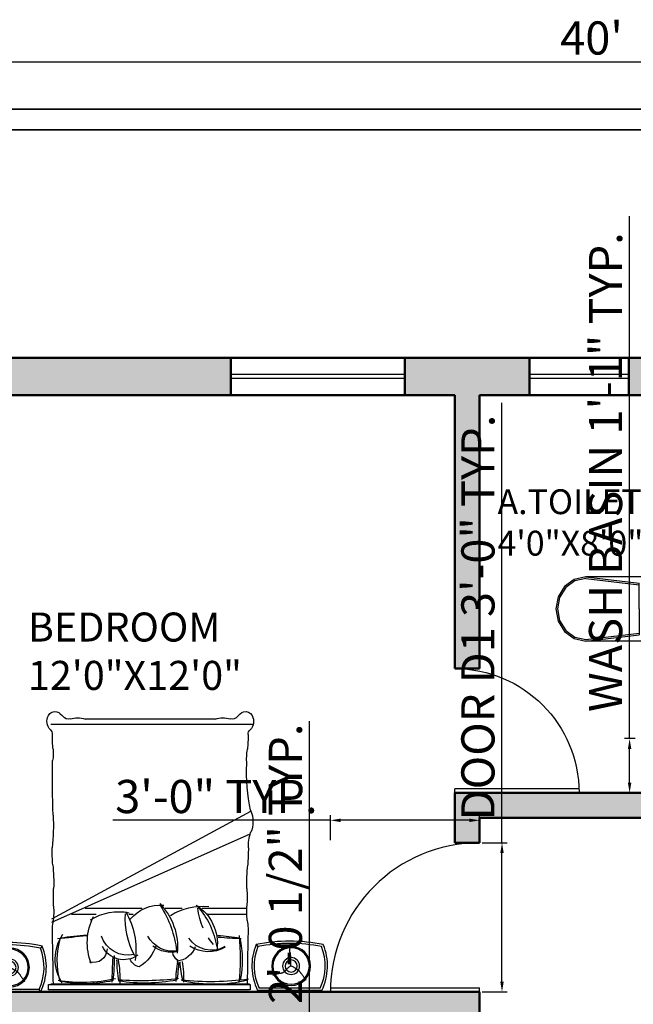
# Model space of a CAD drawing. Units: inches. Extents: x 3008 to 4088, y 1255 to 2137.
# Tile 27 of 30: x 3705 to 3853, y 1794 to 2031. Entities that reach past the tile are written whole.
import ezdxf

# ---------------------------------------------------------------- set-up
doc = ezdxf.new("R2010")
doc.units = ezdxf.units.IN
for name, color, linetype, lineweight in [('A-ANNO-DIMS', 2, 'Continuous', 18), ('A-AREA-IDEN', 7, 'Continuous', 18), ('A-DOOR', 4, 'Continuous', 25), ('A-FLOR-FIXT', 8, 'Continuous', 18), ('A-FURN', 8, 'Continuous', 18), ('A-GLAZ', 4, 'Continuous', 25), ('A-WALL', 7, 'Continuous', 50), ('A-WALL-PATT', 8, 'Continuous', 13), ('C-PROP', 1, 'Continuous', 35)]:
    doc.layers.add(name, color=color, linetype=linetype, lineweight=lineweight)
doc.layers.add('SANTEH', color=7, linetype='Continuous')
doc.layers.add('TEFRİŞ', color=11, linetype='Continuous')
doc.styles.get("Standard").update_dxf_attribs({"font": 'arial.ttf'})
doc.dimstyles.new('ISO-25', dxfattribs={"dimtxt": 8, "dimasz": 2.5, "dimexe": 1.25, "dimexo": 0.625, "dimtad": 1, "dimdec": 1, "dimlunit": 3, "dimtxsty": 'Standard', "dimcen": 2.5, "dimadec": 0, "dimazin": 0, "dimtfac": 1, "dimtdec": 1, "dimtmove": 0, "dimatfit": 3, "dimfxl": 1, "dimarcsym": 0})

# ---------------------------------------------------------------- blocks, each defined once
blk = doc.blocks.new('*D31')
at = {"layer": 'A-ANNO-DIMS', "color": 0, "lineweight": -2, "transparency": 16777216}
for p, q in [((3602.94, 2010.35), (3602.94, 2022.41)), ((4082.94, 2010.35), (4082.94, 2022.41)), ((3605.44, 2021.16), (4080.44, 2021.16))]:
    blk.add_line(p, q, dxfattribs=at)
at = {"layer": 'A-ANNO-DIMS', "color": 0, "transparency": 16777216}
for points in [[(3605.44, 2021.58), (3605.44, 2020.74), (3602.94, 2021.16)], [(4080.44, 2021.58), (4080.44, 2020.74), (4082.94, 2021.16)]]:
    blk.add_solid(points, dxfattribs=at)
at = {"layer": 'Defpoints', "color": 0, "transparency": 16777216}
for p in [(4082.94, 2021.16), (3602.94, 2009.72), (4082.94, 2009.72)]:
    blk.add_point(p, dxfattribs=at)
at = {"layer": 'A-ANNO-DIMS', "color": 0, "transparency": 16777216, "insert": (3842.94, 2025.87), "char_height": 8, "attachment_point": 5}
blk.add_mtext("40'", dxfattribs=at)
blk = doc.blocks.new('D2')
for p, q in [((1722.5, 1505.46), (1722.5, 1475.46)), ((1723.5, 1505.46), (1723.5, 1475.46)), ((1722.5, 1475.46), (1723.5, 1475.46))]:
    blk.add_line(p, q)
blk.add_arc((1722.5, 1475.46), 30, 0, 90)
blk = doc.blocks.new('D1')
for p, q in [((1805.96, 1500.36), (1805.96, 1464.36)), ((1806.96, 1500.36), (1806.96, 1464.36)), ((1805.96, 1464.36), (1806.96, 1464.36))]:
    blk.add_line(p, q)
blk.add_arc((1805.96, 1464.36), 36, 0, 90)
blk = doc.blocks.new('WC 2 Symb_109')
at = {"layer": 'SANTEH'}
for p, q in [((0, 0), (0, 380)), ((0, 380), (132.4, 380)), ((153.6, 364.9), (506.8, 364.9)), ((506.3, 364.9), (215.7, 330.9)), ((506.3, 356), (215.7, 322)), ((215.7, 190), (215.7, 330.9)), ((215.7, 190), (215.7, 49.1)), ((506.3, 24), (215.7, 58)), ((153.8, 15.1), (506.8, 15.1)), ((506.3, 15.1), (215.7, 49.1)), ((0, 0), (132.4, 0))]:
    blk.add_line(p, q, dxfattribs=at)
for points in [[(154.6, 360.1), (153.9, 364.1), (152.3, 367.9), (150.2, 371.3), (147.4, 374.3), (144.1, 376.7), (140.5, 378.5), (136.5, 379.6), (132.4, 380)], [(154.6, 19.7), (158.6, 62.1), (161.4, 104.7), (163.1, 147.3), (163.7, 189.9), (163.1, 232.5), (161.4, 275.1), (158.6, 317.7), (154.6, 360.1)], [(506.3, 24), (565.5, 36.6), (615.7, 72.6), (649.2, 126.5), (661, 190), (649.2, 253.5), (615.7, 307.4), (565.5, 343.4), (506.3, 356)], [(506.8, 15.1), (569.2, 28.4), (622.2, 66.3), (657.6, 123.1), (670, 190), (657.6, 256.9), (622.2, 313.7), (569.2, 351.6), (506.8, 364.9)], [(132.4, 0), (136.5, 0.4), (140.4, 1.5), (144.1, 3.2), (147.3, 5.6), (150.1, 8.6), (152.3, 12), (153.8, 15.7), (154.6, 19.7)]]:
    blk.add_lwpolyline(points, dxfattribs=at)
blk.add_lwpolyline([(83.6, 208.5), (70.4, 203.1), (64.9, 190), (70.4, 176.9), (83.6, 171.5), (96.8, 176.9), (102.2, 190), (96.8, 203.1)], close=True, dxfattribs=at)
blk = doc.blocks.new('BED')
at = {"layer": 'TEFRİŞ'}
for p, q in [((2114.88, 1835.66), (2129.12, 1835.66)), ((2115.2, 1835.15), (2128.8, 1835.15)), ((2130.81, 1834.34), (2130.81, 1835.55)), ((2175.56, 1834.34), (2130.81, 1834.34)), ((2130.91, 1835.55), (2175.56, 1835.55)), ((2175, 1834.19), (2130.91, 1834.19)), ((2175.56, 1835.55), (2175.56, 1834.34)), ((2177.29, 1835.98), (2177.61, 1835.47)), ((2177.29, 1835.98), (2191.52, 1835.98)), ((2177.61, 1835.47), (2191.2, 1835.47)), ((2191.2, 1835.47), (2191.52, 1835.98)), ((2118.49, 1833.2), (2118.34, 1833.38)), ((2118.49, 1833.2), (2118.34, 1833.38)), ((2118.63, 1833.03), (2118.49, 1833.2)), ((2118.63, 1833.03), (2118.49, 1833.2)), ((2118.75, 1832.88), (2118.63, 1833.03)), ((2118.75, 1832.88), (2118.63, 1833.03)), ((2118.86, 1832.74), (2118.75, 1832.88)), ((2118.86, 1832.74), (2118.75, 1832.88)), ((2118.95, 1832.61), (2118.86, 1832.74)), ((2118.95, 1832.61), (2118.86, 1832.74)), ((2119.04, 1832.48), (2118.95, 1832.61)), ((2119.04, 1832.48), (2118.95, 1832.61)), ((2119.12, 1832.37), (2119.04, 1832.48)), ((2119.12, 1832.37), (2119.04, 1832.48)), ((2119.19, 1832.26), (2119.12, 1832.37)), ((2119.19, 1832.26), (2119.12, 1832.37)), ((2119.26, 1832.16), (2119.19, 1832.26)), ((2119.26, 1832.16), (2119.19, 1832.26)), ((2119.32, 1832.06), (2119.26, 1832.16)), ((2119.32, 1832.06), (2119.26, 1832.16)), ((2119.39, 1831.97), (2119.32, 1832.06)), ((2119.39, 1831.97), (2119.32, 1832.06)), ((2119.45, 1831.89), (2119.39, 1831.97)), ((2119.45, 1831.89), (2119.39, 1831.97)), ((2124.49, 1831.94), (2124.56, 1831.95)), ((2124.49, 1831.94), (2124.56, 1831.95)), ((2124.56, 1831.95), (2124.64, 1831.96)), ((2124.56, 1831.95), (2124.64, 1831.96)), ((2124.64, 1831.96), (2124.71, 1831.98)), ((2124.64, 1831.96), (2124.71, 1831.98)), ((2124.71, 1831.98), (2124.79, 1831.99)), ((2124.71, 1831.98), (2124.79, 1831.99)), ((2124.79, 1831.99), (2124.87, 1832.01)), ((2124.79, 1831.99), (2124.87, 1832.01)), ((2124.87, 1832.01), (2124.96, 1832.03)), ((2124.87, 1832.01), (2124.96, 1832.03)), ((2124.96, 1832.03), (2125.05, 1832.05)), ((2124.96, 1832.03), (2125.05, 1832.05)), ((2125.05, 1832.05), (2125.14, 1832.08)), ((2125.05, 1832.05), (2125.14, 1832.08)), ((2125.14, 1832.08), (2125.23, 1832.11)), ((2125.14, 1832.08), (2125.23, 1832.11)), ((2125.23, 1832.11), (2125.33, 1832.14)), ((2125.23, 1832.11), (2125.33, 1832.14)), ((2125.33, 1832.14), (2125.42, 1832.17)), ((2125.33, 1832.14), (2125.42, 1832.17)), ((2125.42, 1832.17), (2125.52, 1832.21)), ((2125.42, 1832.17), (2125.52, 1832.21)), ((2125.52, 1832.21), (2125.6, 1832.25)), ((2125.52, 1832.21), (2125.6, 1832.25)), ((2125.6, 1832.25), (2125.68, 1832.3)), ((2125.6, 1832.25), (2125.68, 1832.3)), ((2125.68, 1832.3), (2125.75, 1832.35)), ((2125.68, 1832.3), (2125.75, 1832.35)), ((2180.9, 1833.52), (2180.75, 1833.7)), ((2180.9, 1833.52), (2180.75, 1833.7)), ((2181.04, 1833.35), (2180.9, 1833.52)), ((2181.04, 1833.35), (2180.9, 1833.52)), ((2181.16, 1833.2), (2181.04, 1833.35)), ((2181.16, 1833.2), (2181.04, 1833.35)), ((2181.26, 1833.06), (2181.16, 1833.2)), ((2181.26, 1833.06), (2181.16, 1833.2)), ((2181.36, 1832.93), (2181.26, 1833.06)), ((2181.36, 1832.93), (2181.26, 1833.06)), ((2181.44, 1832.8), (2181.36, 1832.93)), ((2181.44, 1832.8), (2181.36, 1832.93)), ((2181.52, 1832.69), (2181.44, 1832.8)), ((2181.52, 1832.69), (2181.44, 1832.8)), ((2181.59, 1832.58), (2181.52, 1832.69)), ((2181.59, 1832.58), (2181.52, 1832.69)), ((2181.66, 1832.48), (2181.59, 1832.58)), ((2181.66, 1832.48), (2181.59, 1832.58)), ((2181.73, 1832.38), (2181.66, 1832.48)), ((2181.73, 1832.38), (2181.66, 1832.48)), ((2181.79, 1832.29), (2181.73, 1832.38)), ((2181.79, 1832.29), (2181.73, 1832.38)), ((2181.85, 1832.21), (2181.79, 1832.29)), ((2181.85, 1832.21), (2181.79, 1832.29)), ((2181.92, 1832.13), (2181.85, 1832.21)), ((2181.92, 1832.13), (2181.85, 1832.21)), ((2181.97, 1832.05), (2181.92, 1832.13)), ((2181.97, 1832.05), (2181.92, 1832.13)), ((2182.03, 1831.97), (2181.97, 1832.05)), ((2182.03, 1831.97), (2181.97, 1832.05)), ((2182.09, 1831.9), (2182.03, 1831.97)), ((2182.09, 1831.9), (2182.03, 1831.97)), ((2185.68, 1831.9), (2185.75, 1831.95)), ((2185.68, 1831.9), (2185.75, 1831.95)), ((2185.75, 1831.95), (2185.82, 1831.99)), ((2185.75, 1831.95), (2185.82, 1831.99)), ((2185.82, 1831.99), (2185.89, 1832.03)), ((2185.82, 1831.99), (2185.89, 1832.03)), ((2185.89, 1832.03), (2185.96, 1832.06)), ((2185.89, 1832.03), (2185.96, 1832.06)), ((2185.96, 1832.06), (2186.03, 1832.09)), ((2185.96, 1832.06), (2186.03, 1832.09)), ((2186.03, 1832.09), (2186.1, 1832.12)), ((2186.03, 1832.09), (2186.1, 1832.12)), ((2186.1, 1832.12), (2186.17, 1832.14)), ((2186.1, 1832.12), (2186.17, 1832.14)), ((2186.17, 1832.14), (2186.24, 1832.16)), ((2186.17, 1832.14), (2186.24, 1832.16)), ((2186.24, 1832.16), (2186.32, 1832.18)), ((2186.24, 1832.16), (2186.32, 1832.18)), ((2186.32, 1832.18), (2186.39, 1832.19)), ((2186.32, 1832.18), (2186.39, 1832.19)), ((2186.39, 1832.19), (2186.46, 1832.21)), ((2186.39, 1832.19), (2186.46, 1832.21)), ((2186.46, 1832.21), (2186.53, 1832.22)), ((2186.46, 1832.21), (2186.53, 1832.22)), ((2186.53, 1832.22), (2186.61, 1832.23)), ((2186.53, 1832.22), (2186.61, 1832.23)), ((2186.61, 1832.23), (2186.68, 1832.23)), ((2186.61, 1832.23), (2186.68, 1832.23)), ((2186.68, 1832.23), (2186.75, 1832.24)), ((2186.68, 1832.23), (2186.75, 1832.24)), ((2186.75, 1832.24), (2186.82, 1832.25)), ((2186.75, 1832.24), (2186.82, 1832.25)), ((2186.82, 1832.25), (2186.9, 1832.26)), ((2186.82, 1832.25), (2186.9, 1832.26)), ((2186.9, 1832.26), (2186.97, 1832.27)), ((2186.9, 1832.26), (2186.97, 1832.27)), ((2186.97, 1832.27), (2187.04, 1832.28)), ((2186.97, 1832.27), (2187.04, 1832.28)), ((2187.04, 1832.28), (2187.12, 1832.3)), ((2187.04, 1832.28), (2187.12, 1832.3)), ((2187.12, 1832.3), (2187.2, 1832.31)), ((2187.12, 1832.3), (2187.2, 1832.31)), ((2187.2, 1832.31), (2187.28, 1832.33)), ((2187.2, 1832.31), (2187.28, 1832.33)), ((2187.28, 1832.33), (2187.36, 1832.35)), ((2187.28, 1832.33), (2187.36, 1832.35)), ((2187.36, 1832.35), (2187.45, 1832.37)), ((2187.36, 1832.35), (2187.45, 1832.37)), ((2187.45, 1832.37), (2187.54, 1832.4)), ((2187.45, 1832.37), (2187.54, 1832.4)), ((2187.54, 1832.4), (2187.64, 1832.43)), ((2187.54, 1832.4), (2187.64, 1832.43)), ((2187.64, 1832.43), (2187.74, 1832.46)), ((2187.64, 1832.43), (2187.74, 1832.46)), ((2187.74, 1832.46), (2187.83, 1832.49)), ((2187.74, 1832.46), (2187.83, 1832.49)), ((2187.83, 1832.49), (2187.92, 1832.53)), ((2187.83, 1832.49), (2187.92, 1832.53)), ((2187.92, 1832.53), (2188.01, 1832.57)), ((2187.92, 1832.53), (2188.01, 1832.57)), ((2188.01, 1832.57), (2188.09, 1832.62)), ((2188.01, 1832.57), (2188.09, 1832.62)), ((2188.09, 1832.62), (2188.15, 1832.67)), ((2188.09, 1832.62), (2188.15, 1832.67)), ((2119.51, 1831.81), (2119.45, 1831.89)), ((2119.51, 1831.81), (2119.45, 1831.89)), ((2119.57, 1831.73), (2119.51, 1831.81)), ((2119.57, 1831.73), (2119.51, 1831.81)), ((2119.63, 1831.65), (2119.57, 1831.73)), ((2119.63, 1831.65), (2119.57, 1831.73)), ((2119.69, 1831.58), (2119.63, 1831.65)), ((2119.69, 1831.58), (2119.63, 1831.65)), ((2119.75, 1831.51), (2119.69, 1831.58)), ((2119.75, 1831.51), (2119.69, 1831.58)), ((2119.81, 1831.44), (2119.75, 1831.51)), ((2119.81, 1831.44), (2119.75, 1831.51)), ((2119.87, 1831.38), (2119.81, 1831.44)), ((2119.87, 1831.38), (2119.81, 1831.44)), ((2119.93, 1831.31), (2119.87, 1831.38)), ((2119.93, 1831.31), (2119.87, 1831.38)), ((2119.99, 1831.25), (2119.93, 1831.31)), ((2119.99, 1831.25), (2119.93, 1831.31)), ((2120.05, 1831.2), (2119.99, 1831.25)), ((2120.05, 1831.2), (2119.99, 1831.25)), ((2120.12, 1831.14), (2120.05, 1831.2)), ((2120.12, 1831.14), (2120.05, 1831.2)), ((2120.18, 1831.09), (2120.12, 1831.14)), ((2120.18, 1831.09), (2120.12, 1831.14)), ((2120.25, 1831.04), (2120.18, 1831.09)), ((2120.25, 1831.04), (2120.18, 1831.09)), ((2120.32, 1830.99), (2120.25, 1831.04)), ((2120.32, 1830.99), (2120.25, 1831.04)), ((2120.39, 1830.94), (2120.32, 1830.99)), ((2120.39, 1830.94), (2120.32, 1830.99)), ((2120.47, 1830.9), (2120.39, 1830.94)), ((2120.47, 1830.9), (2120.39, 1830.94)), ((2120.54, 1830.85), (2120.47, 1830.9)), ((2120.54, 1830.85), (2120.47, 1830.9)), ((2120.62, 1830.8), (2120.54, 1830.85)), ((2120.62, 1830.8), (2120.54, 1830.85)), ((2120.7, 1830.75), (2120.62, 1830.8)), ((2120.7, 1830.75), (2120.62, 1830.8)), ((2120.79, 1830.7), (2120.7, 1830.75)), ((2120.79, 1830.7), (2120.7, 1830.75)), ((2120.88, 1830.65), (2120.79, 1830.7)), ((2120.88, 1830.65), (2120.79, 1830.7)), ((2120.98, 1830.59), (2120.88, 1830.65)), ((2120.98, 1830.59), (2120.88, 1830.65)), ((2121.09, 1830.52), (2120.98, 1830.59)), ((2121.09, 1830.52), (2120.98, 1830.59)), ((2121.21, 1830.45), (2121.09, 1830.52)), ((2121.21, 1830.45), (2121.09, 1830.52)), ((2121.34, 1830.38), (2121.21, 1830.45)), ((2121.34, 1830.38), (2121.21, 1830.45)), ((2121.49, 1830.29), (2121.34, 1830.38)), ((2121.49, 1830.29), (2121.34, 1830.38)), ((2121.66, 1830.21), (2121.49, 1830.29)), ((2121.66, 1830.21), (2121.49, 1830.29)), ((2121.66, 1830.18), (2121.87, 1830.29)), ((2121.66, 1830.18), (2121.87, 1830.29)), ((2121.85, 1830.11), (2121.66, 1830.21)), ((2121.85, 1830.11), (2121.66, 1830.21)), ((2121.74, 1829.99), (2121.73, 1829.83)), ((2121.74, 1829.99), (2121.73, 1829.83)), ((2121.73, 1829.83), (2121.73, 1829.69)), ((2121.73, 1829.83), (2121.73, 1829.69)), ((2121.76, 1830.38), (2121.74, 1830.17)), ((2121.76, 1830.38), (2121.74, 1830.17)), ((2121.74, 1830.17), (2121.74, 1829.99)), ((2121.74, 1830.17), (2121.74, 1829.99)), ((2121.87, 1830.29), (2122.04, 1830.4)), ((2121.87, 1830.29), (2122.04, 1830.4)), ((2122.04, 1830.4), (2122.2, 1830.51)), ((2122.04, 1830.4), (2122.2, 1830.51)), ((2122.2, 1830.51), (2122.33, 1830.61)), ((2122.2, 1830.51), (2122.33, 1830.61)), ((2122.33, 1830.61), (2122.45, 1830.72)), ((2122.33, 1830.61), (2122.45, 1830.72)), ((2122.45, 1830.72), (2122.55, 1830.82)), ((2122.45, 1830.72), (2122.55, 1830.82)), ((2122.55, 1830.82), (2122.64, 1830.91)), ((2122.55, 1830.82), (2122.64, 1830.91)), ((2122.64, 1830.91), (2122.72, 1831.01)), ((2122.64, 1830.91), (2122.72, 1831.01)), ((2122.72, 1831.01), (2122.8, 1831.09)), ((2122.72, 1831.01), (2122.8, 1831.09)), ((2122.8, 1831.09), (2122.87, 1831.18)), ((2122.8, 1831.09), (2122.87, 1831.18)), ((2122.87, 1831.18), (2122.94, 1831.26)), ((2122.87, 1831.18), (2122.94, 1831.26)), ((2122.94, 1831.26), (2123.01, 1831.33)), ((2122.94, 1831.26), (2123.01, 1831.33)), ((2123.01, 1831.33), (2123.08, 1831.4)), ((2123.01, 1831.33), (2123.08, 1831.4)), ((2123.08, 1831.4), (2123.14, 1831.46)), ((2123.08, 1831.4), (2123.14, 1831.46)), ((2123.14, 1831.46), (2123.21, 1831.52)), ((2123.14, 1831.46), (2123.21, 1831.52)), ((2123.21, 1831.52), (2123.27, 1831.58)), ((2123.21, 1831.52), (2123.27, 1831.58)), ((2123.27, 1831.58), (2123.34, 1831.63)), ((2123.27, 1831.58), (2123.34, 1831.63)), ((2123.34, 1831.63), (2123.41, 1831.67)), ((2123.34, 1831.63), (2123.41, 1831.67)), ((2123.41, 1831.67), (2123.48, 1831.71)), ((2123.41, 1831.67), (2123.48, 1831.71)), ((2123.48, 1831.71), (2123.55, 1831.74)), ((2123.48, 1831.71), (2123.55, 1831.74)), ((2123.55, 1831.74), (2123.62, 1831.77)), ((2123.55, 1831.74), (2123.62, 1831.77)), ((2123.62, 1831.77), (2123.69, 1831.8)), ((2123.62, 1831.77), (2123.69, 1831.8)), ((2123.69, 1831.8), (2123.77, 1831.82)), ((2123.69, 1831.8), (2123.77, 1831.82)), ((2123.77, 1831.82), (2123.84, 1831.84)), ((2123.77, 1831.82), (2123.84, 1831.84)), ((2123.84, 1831.84), (2123.91, 1831.86)), ((2123.84, 1831.84), (2123.91, 1831.86)), ((2123.91, 1831.86), (2123.98, 1831.87)), ((2123.91, 1831.86), (2123.98, 1831.87)), ((2123.98, 1831.87), (2124.06, 1831.89)), ((2123.98, 1831.87), (2124.06, 1831.89)), ((2124.06, 1831.89), (2124.13, 1831.9)), ((2124.06, 1831.89), (2124.13, 1831.9)), ((2124.13, 1831.9), (2124.2, 1831.91)), ((2124.13, 1831.9), (2124.2, 1831.91)), ((2124.2, 1831.91), (2124.27, 1831.91)), ((2124.2, 1831.91), (2124.27, 1831.91)), ((2124.27, 1831.91), (2124.35, 1831.92)), ((2124.27, 1831.91), (2124.35, 1831.92)), ((2124.35, 1831.92), (2124.42, 1831.93)), ((2124.35, 1831.92), (2124.42, 1831.93)), ((2124.42, 1831.93), (2124.49, 1831.94)), ((2124.42, 1831.93), (2124.49, 1831.94)), ((2182.15, 1831.83), (2182.09, 1831.9)), ((2182.15, 1831.83), (2182.09, 1831.9)), ((2182.21, 1831.76), (2182.15, 1831.83)), ((2182.21, 1831.76), (2182.15, 1831.83)), ((2182.27, 1831.7), (2182.21, 1831.76)), ((2182.27, 1831.7), (2182.21, 1831.76)), ((2182.33, 1831.63), (2182.27, 1831.7)), ((2182.33, 1831.63), (2182.27, 1831.7)), ((2182.4, 1831.57), (2182.33, 1831.63)), ((2182.4, 1831.57), (2182.33, 1831.63)), ((2182.46, 1831.52), (2182.4, 1831.57)), ((2182.46, 1831.52), (2182.4, 1831.57)), ((2182.52, 1831.46), (2182.46, 1831.52)), ((2182.52, 1831.46), (2182.46, 1831.52)), ((2182.59, 1831.41), (2182.52, 1831.46)), ((2182.59, 1831.41), (2182.52, 1831.46)), ((2182.66, 1831.36), (2182.59, 1831.41)), ((2182.66, 1831.36), (2182.59, 1831.41)), ((2182.73, 1831.31), (2182.66, 1831.36)), ((2182.73, 1831.31), (2182.66, 1831.36)), ((2182.8, 1831.26), (2182.73, 1831.31)), ((2182.8, 1831.26), (2182.73, 1831.31)), ((2182.87, 1831.22), (2182.8, 1831.26)), ((2182.87, 1831.22), (2182.8, 1831.26)), ((2182.95, 1831.17), (2182.87, 1831.22)), ((2182.95, 1831.17), (2182.87, 1831.22)), ((2183.03, 1831.12), (2182.95, 1831.17)), ((2183.03, 1831.12), (2182.95, 1831.17)), ((2183.11, 1831.07), (2183.03, 1831.12)), ((2183.11, 1831.07), (2183.03, 1831.12)), ((2183.2, 1831.02), (2183.11, 1831.07)), ((2183.2, 1831.02), (2183.11, 1831.07)), ((2183.29, 1830.97), (2183.2, 1831.02)), ((2183.29, 1830.97), (2183.2, 1831.02)), ((2183.39, 1830.91), (2183.29, 1830.97)), ((2183.39, 1830.91), (2183.29, 1830.97)), ((2183.49, 1830.84), (2183.39, 1830.91)), ((2183.49, 1830.84), (2183.39, 1830.91)), ((2183.61, 1830.77), (2183.49, 1830.84)), ((2183.61, 1830.77), (2183.49, 1830.84)), ((2183.75, 1830.7), (2183.61, 1830.77)), ((2183.75, 1830.7), (2183.61, 1830.77)), ((2183.9, 1830.61), (2183.75, 1830.7)), ((2183.9, 1830.61), (2183.75, 1830.7)), ((2184.06, 1830.53), (2183.9, 1830.61)), ((2184.06, 1830.53), (2183.9, 1830.61)), ((2184.25, 1830.43), (2184.06, 1830.53)), ((2184.25, 1830.43), (2184.06, 1830.53)), ((2184.07, 1830.5), (2184.27, 1830.61)), ((2184.07, 1830.5), (2184.27, 1830.61)), ((2184.15, 1830.49), (2184.14, 1830.31)), ((2184.15, 1830.49), (2184.14, 1830.31)), ((2184.14, 1830.31), (2184.14, 1830.15)), ((2184.14, 1830.31), (2184.14, 1830.15)), ((2184.14, 1830.15), (2184.14, 1830.01)), ((2184.14, 1830.15), (2184.14, 1830.01)), ((2184.14, 1830.01), (2184.14, 1829.89)), ((2184.14, 1830.01), (2184.14, 1829.89)), ((2184.14, 1829.89), (2184.14, 1829.77)), ((2184.14, 1829.89), (2184.14, 1829.77)), ((2184.14, 1829.77), (2184.14, 1829.67)), ((2184.14, 1829.77), (2184.14, 1829.67)), ((2184.17, 1830.7), (2184.15, 1830.49)), ((2184.17, 1830.7), (2184.15, 1830.49)), ((2184.27, 1830.61), (2184.45, 1830.72)), ((2184.27, 1830.61), (2184.45, 1830.72)), ((2184.45, 1830.72), (2184.6, 1830.83)), ((2184.45, 1830.72), (2184.6, 1830.83)), ((2184.6, 1830.83), (2184.74, 1830.93)), ((2184.6, 1830.83), (2184.74, 1830.93)), ((2184.74, 1830.93), (2184.85, 1831.04)), ((2184.74, 1830.93), (2184.85, 1831.04)), ((2184.85, 1831.04), (2184.95, 1831.14)), ((2184.85, 1831.04), (2184.95, 1831.14)), ((2184.95, 1831.14), (2185.05, 1831.23)), ((2184.95, 1831.14), (2185.05, 1831.23)), ((2185.05, 1831.23), (2185.13, 1831.33)), ((2185.05, 1831.23), (2185.13, 1831.33)), ((2185.13, 1831.33), (2185.21, 1831.41)), ((2185.13, 1831.33), (2185.21, 1831.41)), ((2185.21, 1831.41), (2185.28, 1831.5)), ((2185.21, 1831.41), (2185.28, 1831.5)), ((2185.28, 1831.5), (2185.35, 1831.58)), ((2185.28, 1831.5), (2185.35, 1831.58)), ((2185.35, 1831.58), (2185.42, 1831.65)), ((2185.35, 1831.58), (2185.42, 1831.65)), ((2185.42, 1831.65), (2185.48, 1831.72)), ((2185.42, 1831.65), (2185.48, 1831.72)), ((2185.48, 1831.72), (2185.55, 1831.78)), ((2185.48, 1831.72), (2185.55, 1831.78)), ((2185.55, 1831.78), (2185.61, 1831.84)), ((2185.55, 1831.78), (2185.61, 1831.84)), ((2185.61, 1831.84), (2185.68, 1831.9)), ((2185.61, 1831.84), (2185.68, 1831.9)), ((2121.73, 1829.69), (2121.73, 1829.57)), ((2121.73, 1829.69), (2121.73, 1829.57)), ((2121.73, 1829.57), (2121.73, 1829.45)), ((2121.73, 1829.57), (2121.73, 1829.45)), ((2121.73, 1829.45), (2121.74, 1829.35)), ((2121.73, 1829.45), (2121.74, 1829.35)), ((2121.74, 1828.89), (2121.73, 1828.8)), ((2121.74, 1828.89), (2121.73, 1828.8)), ((2121.73, 1828.8), (2121.73, 1828.72)), ((2121.73, 1828.8), (2121.73, 1828.72)), ((2121.73, 1828.72), (2121.73, 1828.64)), ((2121.73, 1828.72), (2121.73, 1828.64)), ((2121.73, 1828.64), (2121.73, 1828.56)), ((2121.73, 1828.64), (2121.73, 1828.56)), ((2121.73, 1828.56), (2121.73, 1828.48)), ((2121.73, 1828.56), (2121.73, 1828.48)), ((2121.73, 1828.48), (2121.73, 1828.4)), ((2121.73, 1828.48), (2121.73, 1828.4)), ((2121.73, 1828.4), (2121.73, 1828.33)), ((2121.73, 1828.4), (2121.73, 1828.33)), ((2121.73, 1828.33), (2121.74, 1828.25)), ((2121.73, 1828.33), (2121.74, 1828.25)), ((2121.74, 1829.35), (2121.74, 1829.25)), ((2121.74, 1829.35), (2121.74, 1829.25)), ((2121.74, 1829.25), (2121.74, 1829.16)), ((2121.74, 1829.25), (2121.74, 1829.16)), ((2121.74, 1829.16), (2121.74, 1829.06)), ((2121.74, 1829.16), (2121.74, 1829.06)), ((2121.74, 1829.06), (2121.74, 1828.97)), ((2121.74, 1829.06), (2121.74, 1828.97)), ((2121.74, 1828.97), (2121.74, 1828.89)), ((2121.74, 1828.97), (2121.74, 1828.89)), ((2121.74, 1828.25), (2121.75, 1828.18)), ((2121.74, 1828.25), (2121.75, 1828.18)), ((2121.75, 1828.18), (2121.75, 1828.1)), ((2121.75, 1828.18), (2121.75, 1828.1)), ((2121.75, 1828.1), (2121.76, 1828.03)), ((2121.75, 1828.1), (2121.76, 1828.03)), ((2121.76, 1828.03), (2121.78, 1827.95)), ((2121.76, 1828.03), (2121.78, 1827.95)), ((2121.78, 1827.95), (2121.79, 1827.88)), ((2121.78, 1827.95), (2121.79, 1827.88)), ((2121.79, 1827.88), (2121.8, 1827.8)), ((2121.79, 1827.88), (2121.8, 1827.8)), ((2121.8, 1827.8), (2121.82, 1827.72)), ((2121.8, 1827.8), (2121.82, 1827.72)), ((2121.82, 1827.72), (2121.84, 1827.65)), ((2121.82, 1827.72), (2121.84, 1827.65)), ((2121.84, 1827.65), (2121.85, 1827.57)), ((2121.84, 1827.65), (2121.85, 1827.57)), ((2184.14, 1829.04), (2184.13, 1828.96)), ((2184.14, 1829.04), (2184.13, 1828.96)), ((2184.13, 1828.96), (2184.13, 1828.88)), ((2184.13, 1828.96), (2184.13, 1828.88)), ((2184.13, 1828.88), (2184.13, 1828.8)), ((2184.13, 1828.88), (2184.13, 1828.8)), ((2184.13, 1828.8), (2184.14, 1828.72)), ((2184.13, 1828.8), (2184.14, 1828.72)), ((2184.14, 1829.67), (2184.15, 1829.57)), ((2184.14, 1829.67), (2184.15, 1829.57)), ((2184.15, 1829.38), (2184.14, 1829.29)), ((2184.15, 1829.38), (2184.14, 1829.29)), ((2184.14, 1829.29), (2184.14, 1829.21)), ((2184.14, 1829.29), (2184.14, 1829.21)), ((2184.14, 1829.21), (2184.14, 1829.12)), ((2184.14, 1829.21), (2184.14, 1829.12)), ((2184.14, 1829.12), (2184.14, 1829.04)), ((2184.14, 1829.12), (2184.14, 1829.04)), ((2184.14, 1828.72), (2184.14, 1828.65)), ((2184.14, 1828.72), (2184.14, 1828.65)), ((2184.14, 1828.65), (2184.15, 1828.57)), ((2184.14, 1828.65), (2184.15, 1828.57)), ((2184.15, 1829.57), (2184.15, 1829.48)), ((2184.15, 1829.57), (2184.15, 1829.48)), ((2184.15, 1829.48), (2184.15, 1829.38)), ((2184.15, 1829.48), (2184.15, 1829.38)), ((2184.15, 1828.57), (2184.15, 1828.5)), ((2184.15, 1828.57), (2184.15, 1828.5)), ((2184.15, 1828.5), (2184.16, 1828.42)), ((2184.15, 1828.5), (2184.16, 1828.42)), ((2184.16, 1828.42), (2184.17, 1828.35)), ((2184.16, 1828.42), (2184.17, 1828.35)), ((2184.17, 1828.35), (2184.18, 1828.27)), ((2184.17, 1828.35), (2184.18, 1828.27)), ((2184.18, 1828.27), (2184.19, 1828.2)), ((2184.18, 1828.27), (2184.19, 1828.2)), ((2184.19, 1828.2), (2184.21, 1828.12)), ((2184.19, 1828.2), (2184.21, 1828.12)), ((2184.21, 1828.12), (2184.22, 1828.04)), ((2184.21, 1828.12), (2184.22, 1828.04)), ((2184.22, 1828.04), (2184.24, 1827.97)), ((2184.22, 1828.04), (2184.24, 1827.97)), ((2184.24, 1827.97), (2184.26, 1827.89)), ((2184.24, 1827.97), (2184.26, 1827.89)), ((2184.26, 1827.89), (2184.28, 1827.81)), ((2184.26, 1827.89), (2184.28, 1827.81)), ((2184.28, 1827.81), (2184.3, 1827.73)), ((2184.28, 1827.81), (2184.3, 1827.73)), ((2184.3, 1827.73), (2184.32, 1827.65)), ((2184.3, 1827.73), (2184.32, 1827.65)), ((2184.32, 1827.65), (2184.34, 1827.58)), ((2184.32, 1827.65), (2184.34, 1827.58)), ((2184.34, 1827.58), (2184.36, 1827.5)), ((2184.34, 1827.58), (2184.36, 1827.5)), ((2121.78, 1825.93), (2121.74, 1825.8)), ((2121.78, 1825.93), (2121.74, 1825.8)), ((2121.83, 1826.06), (2121.78, 1825.93)), ((2121.83, 1826.06), (2121.78, 1825.93)), ((2121.87, 1826.19), (2121.83, 1826.06)), ((2121.87, 1826.19), (2121.83, 1826.06)), ((2121.85, 1827.57), (2121.87, 1827.49)), ((2121.85, 1827.57), (2121.87, 1827.49)), ((2121.87, 1827.49), (2121.89, 1827.41)), ((2121.87, 1827.49), (2121.89, 1827.41)), ((2121.91, 1826.31), (2121.87, 1826.19)), ((2121.91, 1826.31), (2121.87, 1826.19)), ((2121.89, 1827.41), (2121.91, 1827.33)), ((2121.89, 1827.41), (2121.91, 1827.33)), ((2121.91, 1827.33), (2121.93, 1827.26)), ((2121.91, 1827.33), (2121.93, 1827.26)), ((2121.95, 1826.42), (2121.91, 1826.31)), ((2121.95, 1826.42), (2121.91, 1826.31)), ((2121.93, 1827.26), (2121.95, 1827.18)), ((2121.93, 1827.26), (2121.95, 1827.18)), ((2121.95, 1827.18), (2121.97, 1827.09)), ((2121.95, 1827.18), (2121.97, 1827.09)), ((2121.97, 1826.54), (2121.95, 1826.42)), ((2121.97, 1826.54), (2121.95, 1826.42)), ((2121.97, 1827.09), (2121.99, 1827.01)), ((2121.97, 1827.09), (2121.99, 1827.01)), ((2121.99, 1826.64), (2121.97, 1826.54)), ((2121.99, 1826.64), (2121.97, 1826.54)), ((2121.99, 1827.01), (2122, 1826.93)), ((2121.99, 1827.01), (2122, 1826.93)), ((2122, 1826.74), (2121.99, 1826.64)), ((2122, 1826.74), (2121.99, 1826.64)), ((2122, 1826.93), (2122.01, 1826.84)), ((2122, 1826.93), (2122.01, 1826.84)), ((2122.01, 1826.84), (2122, 1826.74)), ((2122.01, 1826.84), (2122, 1826.74)), ((2129.46, 1825.49), (2129.09, 1825.93)), ((2176.94, 1825.81), (2177.31, 1826.25)), ((2184.19, 1826.25), (2184.14, 1826.12)), ((2184.19, 1826.25), (2184.14, 1826.12)), ((2184.23, 1826.38), (2184.19, 1826.25)), ((2184.23, 1826.38), (2184.19, 1826.25)), ((2184.28, 1826.51), (2184.23, 1826.38)), ((2184.28, 1826.51), (2184.23, 1826.38)), ((2184.32, 1826.63), (2184.28, 1826.51)), ((2184.32, 1826.63), (2184.28, 1826.51)), ((2184.35, 1826.74), (2184.32, 1826.63)), ((2184.35, 1826.74), (2184.32, 1826.63)), ((2184.38, 1826.86), (2184.35, 1826.74)), ((2184.38, 1826.86), (2184.35, 1826.74)), ((2184.36, 1827.5), (2184.38, 1827.41)), ((2184.36, 1827.5), (2184.38, 1827.41)), ((2184.38, 1827.41), (2184.4, 1827.33)), ((2184.38, 1827.41), (2184.4, 1827.33)), ((2184.4, 1826.96), (2184.38, 1826.86)), ((2184.4, 1826.96), (2184.38, 1826.86)), ((2184.4, 1827.33), (2184.41, 1827.25)), ((2184.4, 1827.33), (2184.41, 1827.25)), ((2184.41, 1827.06), (2184.4, 1826.96)), ((2184.41, 1827.06), (2184.4, 1826.96)), ((2184.41, 1827.25), (2184.41, 1827.16)), ((2184.41, 1827.25), (2184.41, 1827.16)), ((2184.41, 1827.16), (2184.41, 1827.06)), ((2184.41, 1827.16), (2184.41, 1827.06)), ((2191.87, 1825.81), (2191.5, 1826.25)), ((2174.77, 1819.77), (2130.6, 1795.83)), ((2174.77, 1820.53), (2130.76, 1800.91)), ((2140.43, 1818.69), (2131.53, 1818.69)), ((2141.43, 1817.4), (2131.53, 1817.4)), ((2149.62, 1817.4), (2145.88, 1817.4)), ((2167.36, 1817.4), (2154.77, 1817.4)), ((2157.71, 1818.69), (2156.77, 1818.69)), ((2170.41, 1818.69), (2164.92, 1818.69)), ((2175, 1776.57), (2130.11, 1776.57)), ((2138.52, 1775.41), (2167.39, 1775.41))]:
    blk.add_line(p, q, dxfattribs=at)
for centre, radius, start, end in [((2126, 1830.19), 12.39, 153.8162, 202.314), ((2126, 1830.19), 11.88, 155.3335, 201.0157), ((2118, 1830.19), 11.88, 338.9843, 24.6665), ((2118, 1830.19), 12.39, 337.686, 26.1838), ((2188.4, 1830.51), 12.39, 153.8162, 202.314), ((2188.4, 1830.51), 11.88, 155.3335, 201.0157), ((2180.41, 1830.51), 11.88, 338.9843, 24.6665), ((2180.41, 1830.51), 12.39, 337.686, 26.1838), ((2122, 1861.35), 36.63, 258.2443, 281.7557), ((2122, 1861.35), 36.12, 258.6773, 281.3227), ((2184.41, 1861.67), 36.63, 258.2443, 281.7557), ((2184.41, 1861.67), 36.12, 258.6773, 281.3227)]:
    blk.add_arc(centre, radius, start, end, dxfattribs=at)
at = {"layer": 'TEFRİŞ', "extrusion": (0, 0, -1)}
for centre, major_axis, ratio, start_param, end_param in [((2121.68, 1830.24), (-3.05, -3.05), 1, 3.926991, 10.210176), ((2121.68, 1830.24), (2.86, -2.86), 1, 5.497787, 11.780972), ((2121.68, 1830.24), (2.86, -2.86), 1, 5.497787, 11.780972), ((2206.14, 1830.73), (-52.86, -52.86), 1, 0.767743, 0.83177), ((2138.85, 1803.05), (-22.1, 22.1), 1, 0.544604, 1.006234), ((2154.12, 1796.61), (-26.46, 26.46), 1, 0.596409, 0.940188), ((2168.35, 1789.27), (-1.33, 44.62), 0.875277, -0.163954, 0.163954), ((2167.6, 1797.72), (-0.51, 36.47), 0.865194, -0.185965, 0.185965), ((2184.09, 1830.56), (-3.05, -3.05), 1, 3.926991, 10.210176), ((2184.09, 1830.56), (2.86, -2.86), 1, 5.497787, 11.780972), ((2184.09, 1830.56), (2.86, -2.86), 1, 5.497787, 11.780972), ((2121.68, 1830.24), (1.33, -1.33), 1, 5.497787, 11.780972), ((2121.68, 1830.24), (1.33, -1.33), 1, 5.497787, 11.780972), ((2139.43, 1773.84), (-42.35, 42.35), 1, 0.646251, 0.896949), ((2154.7, 1828.89), (-15.68, 15.68), 1, -1.00675, -0.580436), ((2181.61, 1828.44), (-34.39, 34.39), 1, -0.888486, -0.672463), ((2164.51, 1832.79), (-13.41, 13.41), 1, -0.974476, -0.730892), ((2127.6, 1828.81), (-13.23, 13.23), 1, 2.100388, 2.328052), ((2155, 1761.9), (-50.65, -50.65), 1, 2.239512, 2.426533), ((2172.01, 1828.66), (-17.93, 17.93), 1, -0.753394, -0.598744), ((2128.44, 1832.96), (-13.26, -13.26), 1, 3.889049, 4.127298), ((2183.72, 1833.22), (-17, 17), 1, -0.967105, -0.749712), ((2134, 1828.8), (-18.62, 18.62), 1, 2.173461, 2.355043), ((2199.2, 1828.45), (-27.06, -27.06), 1, 0.770625, 0.917228), ((2087.32, 1833.96), (-52.37, 52.37), 1, 2.358049, 2.431787), ((2164.15, 1828.7), (-6.99, 6.99), 1, 1.789136, 2.946702), ((2156.76, 1828.98), (-11.9, -11.9), 1, 3.646453, 4.226155), ((2099.77, 1830.73), (-52.86, 52.86), 1, 2.311571, 2.373849), ((2184.09, 1830.56), (1.33, -1.33), 1, 5.497787, 11.780972), ((2184.09, 1830.56), (1.33, -1.33), 1, 5.497787, 11.780972), ((2184.09, 1830.56), (0.952, -0.952), 1, 5.497787, 11.780972), ((2184.09, 1830.56), (0.952, -0.952), 1, 5.497787, 11.780972), ((2121.68, 1830.24), (0.952, -0.952), 1, 5.497787, 11.780972), ((2121.68, 1830.24), (0.952, -0.952), 1, 5.497787, 11.780972), ((2159.55, 1823.33), (-5.81, 5.81), 1, -0.516587, 0.256776), ((2154.84, 1827.75), (-1.93, 1.93), 1, 0.997904, 1.977819), ((2166.67, 1824.96), (-2.93, 3.91), 0.760601, -0.723751, 0.723751), ((2675.38, 1815.09), (-384.79, -384.79), 1, 0.80103, 0.811711), ((2147.44, 1824.41), (-3.36, -3.36), 1, 1.11934, 2.270556), ((2145.66, 1827.01), (-1.62, 1.62), 1, 1.310976, 2.284591), ((2172, 1826.44), (-11.23, 11.23), 1, -1.332486, -0.624868), ((2158.82, 1823.55), (-3.74, -3.74), 1, 1.730792, 3.47045), ((2141.71, 1819.83), (-11.86, 11.86), 1, 1.850844, 2.42862), ((2157.83, 1821.53), (-4.47, 4.47), 1, 0.576679, 2.021689), ((2153.88, 1825.05), (-9.22, 9.22), 1, 1.994956, 2.818753), ((1630.53, 1815.09), (-384.79, 384.79), 1, 2.329881, 2.340562), ((2140.05, 1819.86), (-5.1, 5.1), 1, 0.238357, 1.390139), ((2139.42, 1820.79), (-4.21, -4.21), 1, 1.82161, 3.349145), ((2148.15, 1825.25), (-7.14, -7.14), 1, 6.061986, 7.190757), ((2154.93, 1828.48), (-11.96, 11.96), 1, -1.530302, -0.934407), ((2127.37, 1815.76), (-10.68, 10.68), 1, 1.657204, 1.779381), ((2160.6, 1825.98), (-9.68, -9.68), 1, 0.009196, 0.886853), ((2148.35, 1820.65), (-4.63, -4.63), 1, 2.117602, 3.020837), ((2147.86, 1820.64), (-4.48, 4.48), 1, 0.665914, 1.867503), ((2170.68, 1829.67), (-16.79, 16.79), 1, -1.354718, -0.902276), ((2146.08, 1822.57), (-10.5, 10.5), 1, -0.951783, -0.716225), ((2132.43, 1774.09), (-35.41, -35.41), 1, 2.362911, 2.464592), ((2140.17, 1862.96), (-27.99, 27.99), 1, 3.983025, 4.107469), ((2165.73, 1860.69), (-26.41, -26.41), 1, 5.306413, 5.463767), ((2199.62, 1529.47), (-209.2, 209.2), 1, 0.675361, 0.697001), ((2159.82, 1822.57), (-10.5, -10.5), 1, 3.857817, 4.093375), ((2127.37, 1815.76), (-10.68, 10.68), 1, 1.94252, 2.248924), ((2111.06, 1818.12), (-14.48, 14.48), 1, 2.258605, 2.412359), ((2141.33, 1830.48), (-9.55, -9.55), 1, 4.941413, 5.601673), ((2150.79, 1825.18), (-6, 6), 1, 3.032122, 4.026148), ((2159.02, 1834.9), (-3.04, 16.53), 0.830169, 2.822117, 3.461068), ((2194.85, 1818.12), (-14.48, 14.48), 1, -0.841563, -0.687809), ((2169.92, 1815.01), (-27.2, -27.2), 1, 0.734393, 0.836404), ((2135.98, 1815.01), (-27.2, -27.2), 1, 3.875985, 3.977996), ((2098.24, 1811.68), (-23.54, -23.54), 1, 3.885834, 4.043401), ((2207.66, 1811.68), (-23.54, -23.54), 1, 0.668988, 0.826555), ((2189.03, 1803.74), (-40.91, -40.91), 1, 0.789771, 0.855756), ((2116.87, 1803.74), (-40.91, 40.91), 1, 2.285836, 2.351822), ((2122.14, 1803.63), (-6.39, -6.39), 1, 3.886359, 4.265474), ((2222.76, 1798.77), (-34.16, -34.16), 1, 0.743488, 0.893627), ((2135.02, 1798.41), (-3.45, 3.45), 1, -0.831635, -0.314979), ((2135.48, 1798), (-3.77, -3.77), 1, 0.329385, 0.820948), ((2127.76, 1790.23), (-1, 12.37), 0.296708, 1.141067, 2.000525), ((2148.06, 1790.38), (-0.75, 67.37), 0.394952, 1.480524, 1.661068), ((2118.49, 1784.2), (-9.24, -9.24), 1, 3.839645, 4.088086), ((2182.27, 1782.99), (-5.52, -5.52), 1, 0.671703, 0.993321), ((2162.12, 1778.86), (-21.85, 21.85), 1, -0.78611, -0.680117), ((2143.78, 1778.86), (-21.85, 21.85), 1, 2.250913, 2.356906), ((2132.72, 1775.92), (-1.91, -1.91), 1, 0.284117, 1.557111), ((2129.83, 1778.8), (-0.986, 0.986), 1, 2.330985, 3.163296), ((2176.08, 1778.8), (-0.986, 0.986), 1, 4.690686, 5.522997), ((2173.18, 1775.92), (-1.91, -1.91), 1, 3.155278, 4.428271), ((2134.73, 1774.06), (-0.964, -0.964), 1, 1.381176, 2.701227), ((2136.75, 1781.14), (-4.24, 4.24), 1, 3.62713, 4.188813), ((2169.16, 1781.14), (-4.24, 4.24), 1, 3.665169, 4.226852), ((2171.17, 1774.06), (-0.964, -0.964), 1, 2.011162, 3.331212), ((2131.79, 1775.28), (-1.11, 1.11), 1, 3.629269, 5.067473), ((2130.83, 1777), (-2.49, -2.49), 1, 4.590984, 5.084038), ((2175.07, 1777), (-2.49, 2.49), 1, 4.34074, 4.833793), ((2174.12, 1775.28), (-1.11, 1.11), 1, 2.786508, 4.224712)]:
    blk.add_ellipse(centre, major_axis=major_axis, ratio=ratio, start_param=start_param, end_param=end_param, dxfattribs=at)
blk = doc.blocks.new('*D39')
at = {"layer": 'A-ANNO-DIMS', "color": 0, "lineweight": -2, "transparency": 16777216}
for p, q in [((3821.34, 1832.72), (3821.34, 1938.86)), ((3816.57, 1832.72), (3822.59, 1832.72)), ((3821.34, 1799.22), (3821.34, 1830.22)), ((3816.57, 1796.72), (3822.59, 1796.72))]:
    blk.add_line(p, q, dxfattribs=at)
at = {"layer": 'A-ANNO-DIMS', "color": 0, "transparency": 16777216}
for points in [[(3820.92, 1830.22), (3821.76, 1830.22), (3821.34, 1832.72)], [(3820.92, 1799.22), (3821.76, 1799.22), (3821.34, 1796.72)]]:
    blk.add_solid(points, dxfattribs=at)
at = {"layer": 'Defpoints', "color": 0, "transparency": 16777216}
for p in [(3815.94, 1832.72), (3821.34, 1832.72), (3815.94, 1796.72)]:
    blk.add_point(p, dxfattribs=at)
at = {"layer": 'A-ANNO-DIMS', "color": 0, "transparency": 16777216, "insert": (3816.57, 1887.04), "char_height": 8, "attachment_point": 5, "rotation": 90}
blk.add_mtext('DOOR D1 3\'-0" TYP.', dxfattribs=at)
blk = doc.blocks.new('*D40')
at = {"layer": 'A-ANNO-DIMS', "color": 0, "lineweight": -2, "transparency": 16777216}
for p, q in [((3779.94, 1833.35), (3779.94, 1839.37)), ((3815.94, 1833.35), (3815.94, 1839.37)), ((3779.94, 1838.12), (3727.43, 1838.12)), ((3813.44, 1838.12), (3782.44, 1838.12))]:
    blk.add_line(p, q, dxfattribs=at)
at = {"layer": 'A-ANNO-DIMS', "color": 0, "transparency": 16777216}
for points in [[(3782.44, 1838.54), (3782.44, 1837.7), (3779.94, 1838.12)], [(3813.44, 1838.54), (3813.44, 1837.7), (3815.94, 1838.12)]]:
    blk.add_solid(points, dxfattribs=at)
at = {"layer": 'Defpoints', "color": 0, "transparency": 16777216}
for p in [(3779.94, 1838.12), (3779.94, 1832.72), (3815.94, 1832.72)]:
    blk.add_point(p, dxfattribs=at)
at = {"layer": 'A-ANNO-DIMS', "color": 0, "transparency": 16777216, "insert": (3752.44, 1842.83), "char_height": 8, "attachment_point": 5}
blk.add_mtext('3\'-0" TYP.', dxfattribs=at)
blk = doc.blocks.new('*D47')
at = {"layer": 'A-ANNO-DIMS', "color": 0, "lineweight": -2, "transparency": 16777216}
for p, q in [((3852.13, 1857.83), (3852.13, 1983.94)), ((3853.47, 1857.83), (3850.88, 1857.83)), ((3852.13, 1847.22), (3852.13, 1855.33)), ((3853.47, 1844.72), (3850.88, 1844.72))]:
    blk.add_line(p, q, dxfattribs=at)
at = {"layer": 'A-ANNO-DIMS', "color": 0, "transparency": 16777216}
for points in [[(3851.71, 1855.33), (3852.54, 1855.33), (3852.13, 1857.83)], [(3851.71, 1847.22), (3852.54, 1847.22), (3852.13, 1844.72)]]:
    blk.add_solid(points, dxfattribs=at)
at = {"layer": 'Defpoints', "color": 0, "transparency": 16777216}
for p in [(3852.13, 1857.83), (3854.09, 1857.83), (3854.09, 1844.72)]:
    blk.add_point(p, dxfattribs=at)
at = {"layer": 'A-ANNO-DIMS', "color": 0, "transparency": 16777216, "insert": (3847.36, 1922.14), "char_height": 8, "attachment_point": 5, "rotation": 90}
blk.add_mtext('WASH BASIN 1\'-1" TYP.', dxfattribs=at)
blk = doc.blocks.new('*D54')
at = {"layer": 'A-ANNO-DIMS', "color": 0, "lineweight": -2, "transparency": 16777216}
for p, q in [((3774.89, 1790.72), (3774.89, 1862.01)), ((3778.73, 1790.72), (3773.64, 1790.72)), ((3774.89, 1768.81), (3774.89, 1788.22)), ((3778.73, 1766.31), (3773.64, 1766.31))]:
    blk.add_line(p, q, dxfattribs=at)
at = {"layer": 'A-ANNO-DIMS', "color": 0, "transparency": 16777216}
for points in [[(3774.47, 1788.22), (3775.3, 1788.22), (3774.89, 1790.72)], [(3774.47, 1768.81), (3775.3, 1768.81), (3774.89, 1766.31)]]:
    blk.add_solid(points, dxfattribs=at)
at = {"layer": 'Defpoints', "color": 0, "transparency": 16777216}
for p in [(3774.89, 1790.72), (3779.35, 1790.72), (3779.35, 1766.31)]:
    blk.add_point(p, dxfattribs=at)
at = {"layer": 'A-ANNO-DIMS', "color": 0, "transparency": 16777216, "insert": (3770.12, 1827.62), "char_height": 8, "attachment_point": 5, "rotation": 90}
blk.add_mtext('2\'-0 1/2" TYP.', dxfattribs=at)

msp = doc.modelspace()

# ---------------------------------------------------------------- hatches: boundary and pattern name
at = {"layer": 'A-WALL-PATT'}
h = msp.add_hatch(color=256, dxfattribs=at)
h.dxf.hatch_style = 1
h.paths.add_polyline_path([(3665.94, 1631.72), (3656.94, 1631.72), (3656.94, 1546.72), (3665.94, 1546.72)])
h.paths.add_polyline_path([(3851.94, 1619.72), (3701.94, 1619.72), (3701.94, 1610.72), (3788.94, 1610.72), (3788.94, 1469.72), (3809.94, 1469.72), (3809.94, 1478.72), (3797.94, 1478.72), (3797.94, 1550.72), (3815.94, 1550.72), (3815.94, 1556.72), (3797.94, 1556.72), (3797.94, 1610.72), (3845.94, 1610.72), (3845.94, 1586.72), (3851.94, 1586.72)])
h.paths.add_polyline_path([(4028.94, 1631.72), (4019.94, 1631.72), (4019.94, 1619.72), (3887.94, 1619.72), (3887.94, 1610.72), (4019.94, 1610.72), (4019.94, 1577.72), (4028.94, 1577.72)])
h.paths.add_polyline_path([(3875.94, 1478.72), (3851.94, 1478.72), (3851.94, 1556.72), (3845.94, 1556.72), (3845.94, 1526.72), (3845.94, 1478.72), (3833.94, 1478.72), (3833.94, 1469.72), (3875.94, 1469.72)])
h.paths.add_polyline_path([(3959.94, 1478.72), (3917.94, 1478.72), (3917.94, 1469.72), (3959.94, 1469.72)])
h.paths.add_polyline_path([(4028.94, 1511.72), (4019.94, 1511.72), (4019.94, 1478.72), (4001.94, 1478.72), (4001.94, 1469.72), (4028.94, 1469.72)])
h.paths.add_polyline_path([(4028.94, 1699.22), (4019.94, 1699.22), (4019.94, 1673.72), (3893.94, 1673.72), (3893.94, 1649.72), (3899.94, 1649.72), (3899.94, 1667.72), (4019.94, 1667.72), (4019.94, 1655.72), (4028.94, 1655.72)])
h.paths.add_polyline_path([(4028.94, 1847.72), (4019.94, 1847.72), (4019.94, 1796.72), (3863.94, 1796.72), (3863.94, 1790.72), (4019.94, 1790.72), (4019.94, 1765.22), (4028.94, 1765.22)])
h.paths.add_polyline_path([(3815.94, 1796.72), (3779.94, 1796.72), (3665.94, 1796.72), (3665.94, 1898.72), (3656.94, 1898.72), (3656.94, 1673.72), (3665.94, 1673.72), (3665.94, 1790.72), (3815.94, 1790.72)])
h.paths.add_polyline_path([(3755.94, 1949.72), (3656.94, 1949.72), (3656.94, 1940.72), (3665.94, 1940.72), (3755.94, 1940.72)])
h.paths.add_polyline_path([(3827.94, 1949.72), (3797.94, 1949.72), (3797.94, 1940.72), (3809.94, 1940.72), (3809.94, 1874.72), (3815.94, 1874.72), (3815.94, 1940.72), (3827.94, 1940.72)])
h.paths.add_polyline_path([(3953.94, 1949.72), (3851.94, 1949.72), (3851.94, 1940.72), (3863.94, 1940.72), (3863.94, 1844.72), (3809.94, 1844.72), (3809.94, 1832.72), (3815.94, 1832.72), (3815.94, 1838.72), (3863.94, 1838.72), (3869.94, 1838.72), (3869.94, 1940.72), (3953.94, 1940.72)])
h.paths.add_polyline_path([(4028.94, 1949.72), (3995.94, 1949.72), (3995.94, 1940.72), (4019.94, 1940.72), (4019.94, 1889.72), (4028.94, 1889.72)])

# ---------------------------------------------------------------- linework, layer by layer
at = {"layer": 'A-GLAZ'}
for p, q in [((3797.94, 1945.72), (3755.94, 1945.72)), ((3797.94, 1944.72), (3755.94, 1944.72)), ((3851.94, 1945.72), (3827.94, 1945.72)), ((3851.94, 1944.72), (3827.94, 1944.72))]:
    msp.add_line(p, q, dxfattribs=at)
at = {"layer": 'A-WALL'}
for p, q in [((3656.94, 1949.72), (4028.94, 1949.72)), ((3755.94, 1940.72), (3755.94, 1949.72)), ((3797.94, 1940.72), (3797.94, 1949.72)), ((3827.94, 1940.72), (3827.94, 1949.72)), ((3851.94, 1940.72), (3851.94, 1949.72)), ((3665.94, 1940.72), (3809.94, 1940.72)), ((3809.94, 1874.72), (3809.94, 1940.72)), ((3815.94, 1940.72), (3863.94, 1940.72)), ((3815.94, 1874.72), (3815.94, 1940.72)), ((3809.94, 1874.72), (3815.94, 1874.72)), ((3809.94, 1844.72), (3863.94, 1844.72)), ((3809.94, 1832.72), (3809.94, 1844.72)), ((3815.94, 1838.72), (3863.94, 1838.72)), ((3815.94, 1832.72), (3815.94, 1838.72)), ((3809.94, 1832.72), (3815.94, 1832.72)), ((3665.94, 1796.72), (3815.94, 1796.72)), ((3815.94, 1790.72), (3815.94, 1796.72))]:
    msp.add_line(p, q, dxfattribs=at)
at = {"layer": 'C-PROP'}
for p, q in [((3602.94, 2009.72), (4082.94, 2009.72)), ((3607.94, 2004.72), (4077.94, 2004.72))]:
    msp.add_line(p, q, dxfattribs=at)

# ---------------------------------------------------------------- block references
at = {"layer": 'A-DOOR', "xscale": -1, "rotation": 270}
msp.add_blockref('D2', (2334.48, 122.22), dxfattribs=at)
at = {"layer": 'A-DOOR', "rotation": 90.00000000000003}
msp.add_blockref('D1', (5280.3, -9.24), dxfattribs=at)
at = {"layer": 'A-FLOR-FIXT', "xscale": 0.0441898926459964, "yscale": 0.0441898926459964, "zscale": 0.0441898926459964, "rotation": 180}
msp.add_blockref('WC 2 Symb_109', (3863.94, 1897.51), dxfattribs=at)
at = {"layer": 'A-FURN', "xscale": 1.086875874800008, "yscale": 1.086875874800008, "zscale": 1.086875874800008, "rotation": 180}
msp.add_blockref('BED', (6076.48, 3792.2), dxfattribs=at)

# ---------------------------------------------------------------- texts
at = {"layer": 'A-AREA-IDEN', "attachment_point": 1}
for s, insert, char_height in [('{\\fTimes New Roman|b0|i0|c0|p18;A.TOILET\\P4\'0"X8\'0"}', (3820.26, 1918), 6), ('{\\fTimes New Roman|b0|i0|c0|p18; BEDROOM\\P 12\'0"X12\'0"}', (3704.83, 1888.26), 7)]:
    msp.add_mtext_dynamic_manual_height_columns(s, width=105.6127, gutter_width=12.5, heights=[0], dxfattribs=dict(at, insert=insert, char_height=char_height))

# ---------------------------------------------------------------- dimensions: what is measured, and where the dimension line sits
at = {"layer": 'A-ANNO-DIMS'}
dim = msp.add_linear_dim(base=(4082.94, 2021.16), p1=(3602.94, 2009.72), p2=(4082.94, 2009.72), dimstyle='ISO-25', override={"dimclrd": 0, "dimclre": 0, "dimclrt": 0}, dxfattribs=at)
dim.commit()
dim.dimension.update_dxf_attribs({"geometry": '*D31', "text_midpoint": (3842.94, 2025.87)})
for base, p1, p2, angle, text, picture, middle in [((3852.13, 1857.83), (3854.09, 1844.72), (3854.09, 1857.83), 90, 'WASH BASIN <> TYP.', '*D47', (3847.36, 1922.14)), ((3821.34, 1832.72), (3815.94, 1796.72), (3815.94, 1832.72), 90, 'DOOR D1 <> TYP.', '*D39', (3816.57, 1887.04)), ((3774.89, 1790.72), (3779.35, 1766.31), (3779.35, 1790.72), 90, '<> TYP.', '*D54', (3770.12, 1827.62)), ((3779.94, 1838.12), (3815.94, 1832.72), (3779.94, 1832.72), 180, '<> TYP.', '*D40', (3752.44, 1842.83))]:
    dim = msp.add_linear_dim(base=base, p1=p1, p2=p2, angle=angle, text=text, dimstyle='ISO-25', override={"dimdec": 1, "dimrnd": 0, "dimzin": 1, "dimlunit": 4, "dimfrac": 2}, dxfattribs=at)
    dim.commit()
    dim.dimension.update_dxf_attribs({"geometry": picture, "text_midpoint": middle})

doc.saveas('drawing.dxf')
